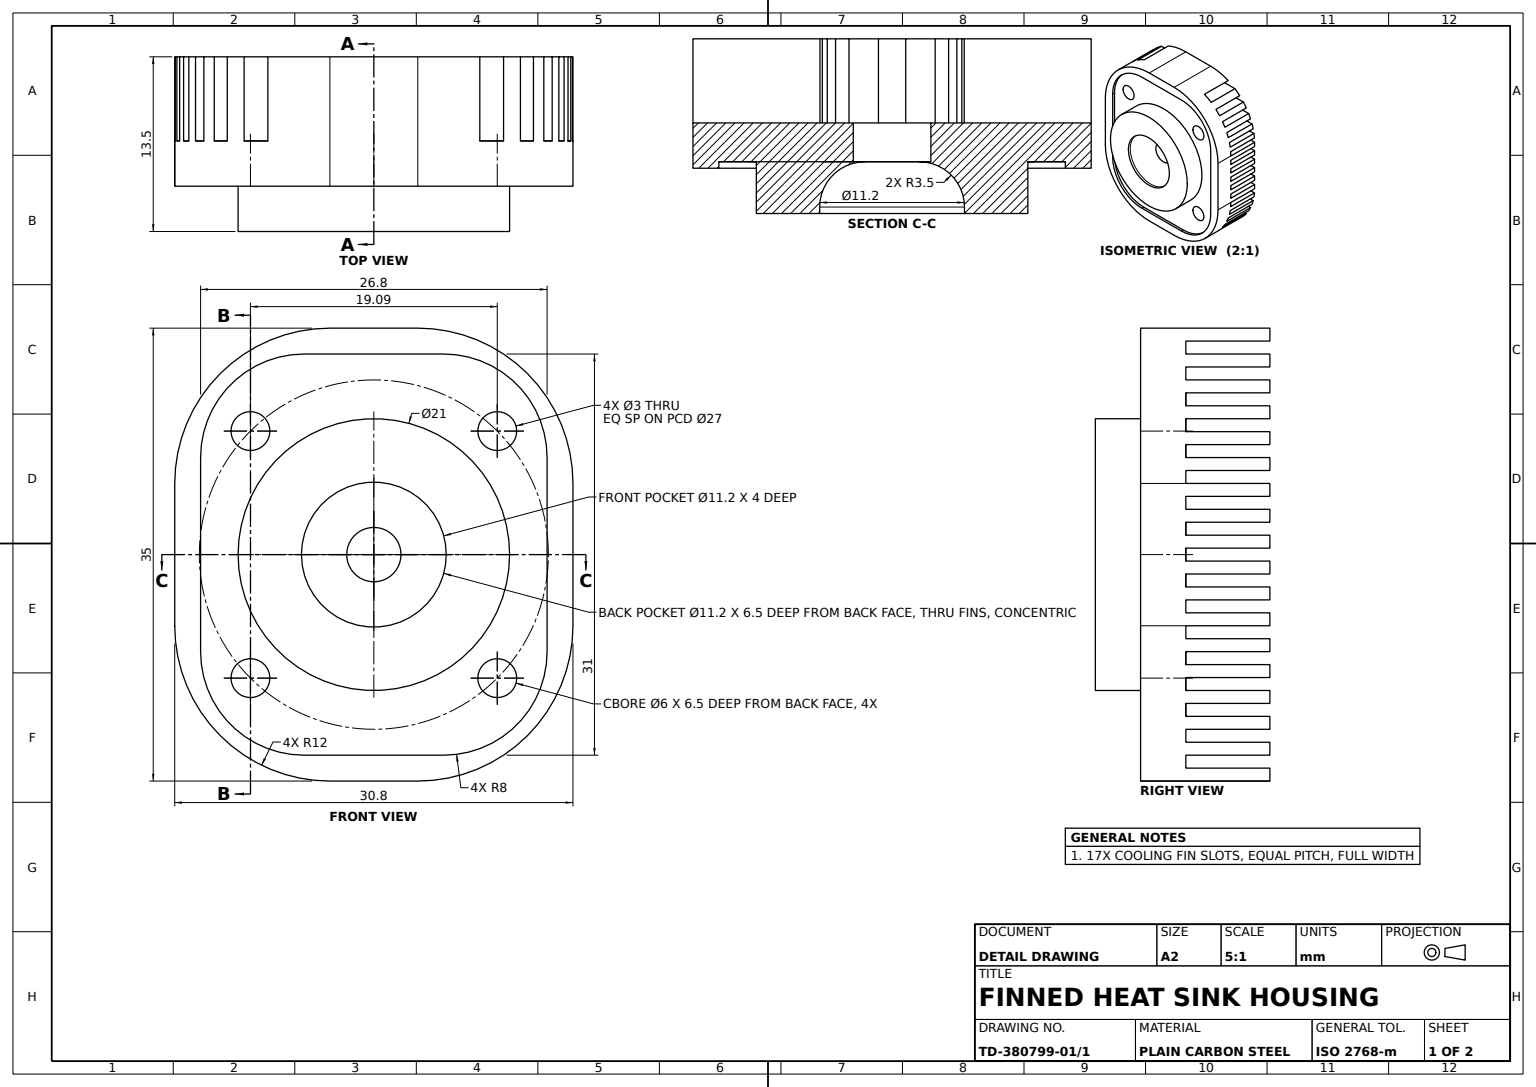
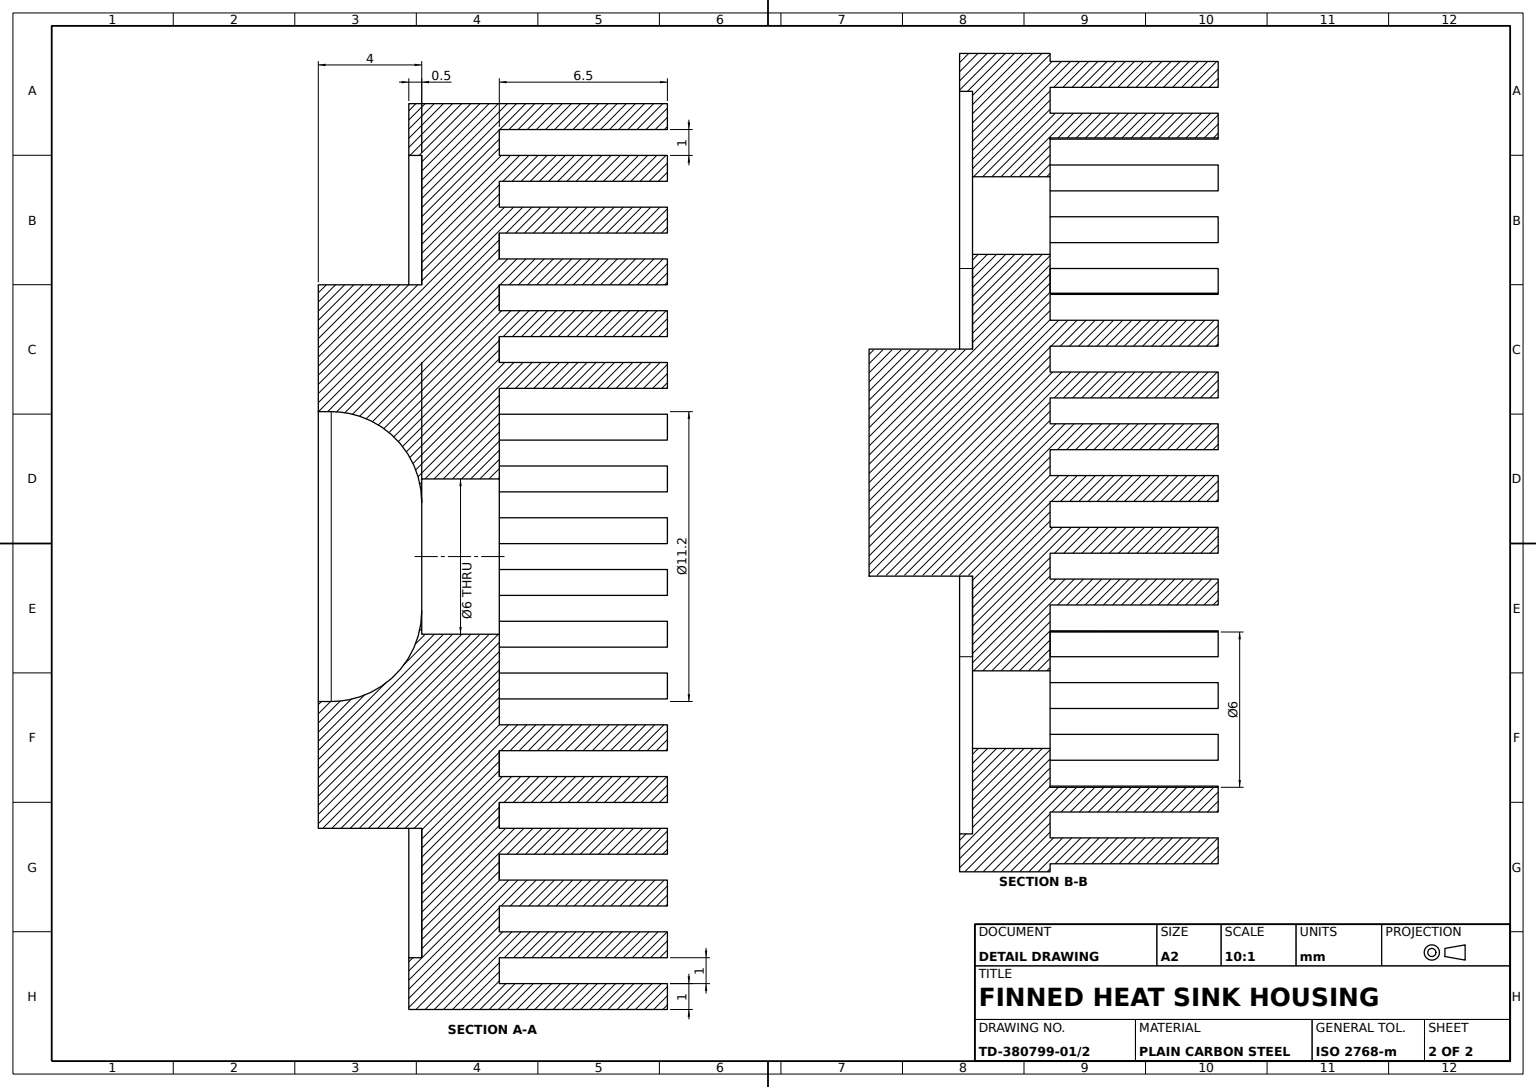
SolidWorks part; units mm, degrees
material "Plain Carbon Steel"
ref_plane "Front Plane" through (0, 0, 0) normal (0, 0, 1) x (1, 0, 0)
ref_plane "Top Plane" through (0, 0, 0) normal (0, 1, 0) x (1, 0, 0)
ref_plane "Right Plane" through (0, 0, 0) normal (1, 0, 0) x (0, 0, -1)
sketch "Head Outline Sketch" plane through (0, 0, 0) normal (0, 0, 1) x (1, 0, 0)
  line L0 (-37.5667, 0) -> (52.1889, 0) construction
  line L1 (0, 25.7833) -> (0, -27.7278) construction
  line L3 (-3.4, -17.5) -> (3.4, -17.5)
  line L4 (-15.4, -5.5) -> (-15.4, 5.5)
  line L5 (-3.4, 17.5) -> (3.4, 17.5)
  line L6 (15.4, -5.5) -> (15.4, 5.5)
  line L7 (-15.4, -17.5) -> (15.4, 17.5) construction
  line L8 (-15.4, 17.5) -> (15.4, -17.5) construction
  arc A0 (-3.4, -17.5) -> (-15.4, -5.5) centre (-3.4, -5.5) cw
  arc A1 (3.4, -17.5) -> (15.4, -5.5) centre (3.4, -5.5) ccw
  arc A2 (3.4, 17.5) -> (15.4, 5.5) centre (3.4, 5.5) cw
  arc A3 (-15.4, 5.5) -> (-3.4, 17.5) centre (-3.4, 5.5) cw
  point P5 (0, 0)
  dimension "D3" = 12
  dimension "D1" = 30.8
  dimension "D2" = 35
extrude "Head Base Body" add sketch "Head Outline Sketch" along normal blind 10
sketch "Face Recess Sketch" plane through (0, 0, 10) normal (0, 0, 1) x (1, 0, 0)
  line L0 (-13.4, 7.5) -> (-13.4, -7.5)
  line L1 (-5.4, -15.5) -> (5.4, -15.5)
  line L2 (13.4, -7.5) -> (13.4, 7.5)
  line L3 (5.4, 15.5) -> (-5.4, 15.5)
  line L4 (15.4, -5.5) -> (15.4, 5.5) construction
  line L5 (-3.4, -17.5) -> (3.4, -17.5) construction
  arc A0 (-5.4, 15.5) -> (-13.4, 7.5) centre (-5.4, 7.5) ccw
  arc A1 (-13.4, -7.5) -> (-5.4, -15.5) centre (-5.4, -7.5) ccw
  arc A2 (5.4, -15.5) -> (13.4, -7.5) centre (5.4, -7.5) ccw
  arc A3 (13.4, 7.5) -> (5.4, 15.5) centre (5.4, 7.5) ccw
  dimension "D1" = 8
  dimension "D2" = 2
  dimension "D3" = 28.8
  dimension "D4" = 2
  dimension "D5" = 33
extrude "Face Recess 0.5mm" cut sketch "Face Recess Sketch" against normal blind 0.5
sketch "Hub Sketch" plane through (0, 0, 9.5) normal (0, 0, 1) x (1, 0, 0)
  circle A0 centre (0, 0) radius 10.5
  circle A1 centre (0, 0) radius 5.6
  dimension "D1" = 21
  dimension "D2" = 11.2
extrude "Raised Hub Ø21" add sketch "Hub Sketch" along normal blind 4
fillet "Recess Fillet R3.5" radius 3.5 1 edges at (5.6, 0, 9.5)
sketch "Centre Bore Sketch" plane through (0, 0, 9.5) normal (0, 0, 1) x (1, 0, 0)
  circle A0 centre (0, 0) radius 3
  dimension "D1" = 6
extrude "Centre Bore Ø6" cut sketch "Centre Bore Sketch" against normal blind 3.5
sketch "Cooling Fin Slots Sketch" plane through (0, 0, 0) normal (1, 0, 0) x (0, 0, -1)
  line L0 (-6.5, 21.5849) -> (-6.5, -19.4994) construction
  line L1 (-21.692, 0) -> (13.4896, 0) construction
  line L2 (-6.5, 2.5) -> (0, 2.5)
  line L3 (-6.5, 0.5) -> (0, 0.5)
  line L4 (-6.5, 0.5) -> (-6.5, -0.5)
  line L5 (-6.5, -0.5) -> (0, -0.5)
  line L6 (0, 0.5) -> (0, -0.5)
  line L7 (-6.5, 1.5) -> (0, 1.5)
  line L8 (0, 2.5) -> (0, 1.5)
  line L9 (-6.5, 2.5) -> (-6.5, 1.5)
  line L10 (-6.5, 4.5) -> (0, 4.5)
  line L11 (-6.5, 3.5) -> (0, 3.5)
  line L12 (0, 4.5) -> (0, 3.5)
  line L13 (-6.5, 4.5) -> (-6.5, 3.5)
  line L14 (-6.5, 6.5) -> (0, 6.5)
  line L15 (-6.5, 5.5) -> (0, 5.5)
  line L16 (0, 6.5) -> (0, 5.5)
  line L17 (-6.5, 6.5) -> (-6.5, 5.5)
  line L18 (-6.5, 8.5) -> (0, 8.5)
  line L19 (-6.5, 7.5) -> (0, 7.5)
  line L20 (0, 8.5) -> (0, 7.5)
  line L21 (-6.5, 8.5) -> (-6.5, 7.5)
  line L22 (-6.5, 10.5) -> (0, 10.5)
  line L23 (-6.5, 9.5) -> (0, 9.5)
  line L24 (0, 10.5) -> (0, 9.5)
  line L25 (-6.5, 10.5) -> (-6.5, 9.5)
  line L26 (-6.5, 12.5) -> (0, 12.5)
  line L27 (-6.5, 11.5) -> (0, 11.5)
  line L28 (0, 12.5) -> (0, 11.5)
  line L29 (-6.5, 12.5) -> (-6.5, 11.5)
  line L30 (-6.5, 14.5) -> (0, 14.5)
  line L31 (-6.5, 13.5) -> (0, 13.5)
  line L32 (0, 14.5) -> (0, 13.5)
  line L33 (-6.5, 14.5) -> (-6.5, 13.5)
  line L34 (-6.5, 16.5) -> (0, 16.5)
  line L35 (-6.5, 15.5) -> (0, 15.5)
  line L36 (0, 16.5) -> (0, 15.5)
  line L37 (-6.5, 16.5) -> (-6.5, 15.5)
  dimension "D1" = 6.5
  dimension "D2" = 1
  dimension "D3" = 6.5
  dimension "D5" = 2
  dimension "D4" = 9
extrude "Cooling Fin Slots" cut sketch "Cooling Fin Slots Sketch" against normal through all both and the other way through all
mirror "Cooling Fin Slots Mirror" about plane through (0, 0, 0) normal (0, 1, 0) of "Cooling Fin Slots"
sketch "Mounting Holes Sketch" plane through (0, 0, 9.5) normal (0, 0, 1) x (1, 0, 0)
  line L0 (0, 23.4021) -> (0, -26.0657) construction
  line L1 (-32.3231, 0) -> (25.4485, 0) construction
  circle A0 centre (-9.545, 9.545) radius 1.5
  circle A1 centre (9.545, 9.545) radius 1.5
  circle A2 centre (9.545, -9.545) radius 1.5
  circle A3 centre (-9.545, -9.545) radius 1.5
  dimension "D1" = 3
  dimension "D2" = 3
  dimension "D3" = 19.09
  dimension "D4" = 19.09
extrude "Mounting Holes Ø3" cut sketch "Mounting Holes Sketch" against normal blind 3.5
sketch "Hub Bore Sketch" plane through (0, 0, 6.5) normal (0, 0, -1) x (-1, 0, 0)
  circle A1 centre (0, 0) radius 5.6
  dimension "D2" = 11.2
extrude "Hub Bore Ø11.2" cut sketch "Hub Bore Sketch" along normal through all
sketch "Side Cut Sketch" plane through (0, 0, 6.5) normal (0, 0, -1) x (-1, 0, 0)
  circle A0 centre (-9.545, 9.545) radius 3
  circle A1 centre (9.545, 9.545) radius 3
  circle A2 centre (-9.545, -9.545) radius 3
  circle A3 centre (9.545, -9.545) radius 3
  dimension "D1" = 6
  dimension "D2" = 6
  dimension "D3" = 6
  dimension "D4" = 6
extrude "Side Cut 6x6" cut sketch "Side Cut Sketch" along normal through all
